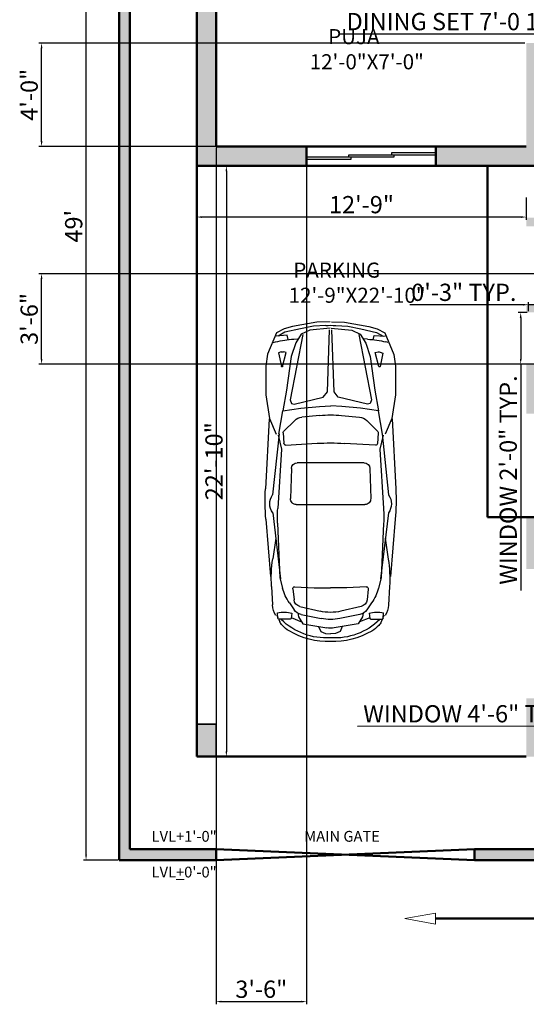
# Model space of a CAD drawing. Units: inches. Extents: x 1913 to 5309, y 1003 to 1733.
# Tile 13 of 23: x 3917 to 4152, y 1032 to 1489. Entities that reach past the tile are written whole.
import ezdxf

# ---------------------------------------------------------------- set-up
doc = ezdxf.new("R2010")
doc.units = ezdxf.units.IN
for name, color, linetype, lineweight in [('A-ANNO-DIMS', 2, 'Continuous', 18), ('A-ANNO-SYMB', 1, 'Continuous', 18), ('A-ANNO-TEXT', 7, 'Continuous', 18), ('A-AREA-IDEN', 3, 'Continuous', 18), ('A-COLS', 5, 'Continuous', 35), ('A-COLS-PATT', 5, 'Continuous', 13), ('A-EQPM', 8, 'Continuous', 18), ('A-FLOR-PATT', 252, 'Continuous', 13), ('A-GLAZ', 5, 'Continuous', 25), ('A-WALL', 7, 'Continuous', 50)]:
    doc.layers.add(name, color=color, linetype=linetype, lineweight=lineweight)
doc.layers.add('L9012X$0', color=2, linetype='Continuous')
doc.styles.get("Standard").update_dxf_attribs({"font": 'arial.ttf'})
doc.dimstyles.new('ISO-25', dxfattribs={"dimtxt": 8, "dimasz": 2.5, "dimexe": 1.25, "dimexo": 0.625, "dimtad": 1, "dimdec": 1, "dimlunit": 3, "dimtxsty": 'Standard', "dimcen": 2.5, "dimclrd": 256, "dimclrt": 1, "dimadec": 0, "dimazin": 0, "dimtfac": 1, "dimtdec": 1, "dimtmove": 0, "dimatfit": 3, "dimfxl": 1, "dimarcsym": 0})

# ---------------------------------------------------------------- blocks, each defined once
blk = doc.blocks.new('*D14')
at = {"layer": 'A-ANNO-DIMS', "color": 0, "lineweight": -2, "transparency": 16777216}
for p, q in [((3962.59, 1686.96), (3946.61, 1686.96)), ((3947.86, 1101.46), (3947.86, 1684.46)), ((3962.59, 1098.96), (3946.61, 1098.96))]:
    blk.add_line(p, q, dxfattribs=at)
at = {"layer": 'A-ANNO-DIMS', "color": 0, "transparency": 16777216}
for points in [[(3947.44, 1684.46), (3948.27, 1684.46), (3947.86, 1686.96)], [(3947.44, 1101.46), (3948.27, 1101.46), (3947.86, 1098.96)]]:
    blk.add_solid(points, dxfattribs=at)
at = {"layer": 'Defpoints', "color": 0, "transparency": 16777216}
for p in [(3947.86, 1686.96), (3963.21, 1686.96), (3963.21, 1098.96)]:
    blk.add_point(p, dxfattribs=at)
at = {"layer": 'A-ANNO-DIMS', "color": 0, "transparency": 16777216, "insert": (3943.15, 1392.96), "char_height": 8, "attachment_point": 5, "rotation": 90}
blk.add_mtext("49'", dxfattribs=at)
blk = doc.blocks.new('A1099DC')
at = {"color": 0, "linetype": 'ByBlock'}
for p, q in [((1279.298465, 804.448389), (2201.430588, 851.890505)), ((2602.736326, 846.078152), (3356.693814, 785.353187)), ((139.051458, 595.027331), (190.951238, 683.213377)), ((179.200345, 564.515703), (190.951238, 709.631982)), ((272.228253, 749.073842), (265.114727, 718.465169)), ((398.733388, 644.315148), (411.280494, 678.748261)), ((411.280494, 678.748261), (588.616917, 641.417897)), ((1482.852352, 674.283145), (1175.286956, 622.180789)), ((1475.52921, 670.226262), (2282.402739, 758.004075)), ((1494.603245, 682.841284), (1678.210958, 641.166865)), ((1678.210958, 641.166865), (2462.684993, 690.847736)), ((2519.280414, 756.817792), (3387.476361, 653.818028)), ((2656.476214, 692.831247), (3376.704709, 662.004075)), ((2851.341839, 715.213377), (3126.60716, 755.701993)), ((3376.704709, 662.004075), (3510.708679, 626.736433)), ((3488.458929, 772.663345), (3732.658862, 759.86454)), ((3909.27561, 688.812956), (3837.725727, 693.401722)), ((3867.794139, 700.329656), (3900.059395, 686.767505)), ((3921.162781, 527.618662), (3921.162781, 676.138994)), ((3925.383812, 676.122818), (3955.306409, 663.545364)), ((92.537504, 388.14361), (139.051458, 595.027331)), ((236.043912, 551.980927), (179.200345, 564.515703)), ((405.405047, 577.538958), (396.874865, 615.894428)), ((589.014326, 626.599587), (405.405047, 577.538958)), ((1300.814287, 466.658131), (1445.712032, 613.104998)), ((1465.665584, 620.56924), (1602.893878, 610.287296)), ((1626.354615, 583.507504), (1602.652901, 169.222264)), ((1933.148906, 509.557888), (2330.980062, 522.200075)), ((3704.596898, 536.993674), (3795.675135, 473.385795)), ((229.117398, 477.634662), (225.714299, 427.957563)), ((1860.238743, -448.635916), (1859.369151, 433.397797)), ((2409.60024, 445.938054), (2410.49349, -460.09121)), ((3493.960271, 465.734554), (3507.923021, 209.166865)), ((3522.252709, 492.345257), (3666.066199, 475.644444)), ((3753.293176, 397.789551), (3815.226005, 132.124765)), ((3839.396146, 426.841284), (3888.358202, 417.538958)), ((3841.786866, 503.451367), (3910.58243, 515.096797)), ((3888.358202, 417.538958), (3983.199613, 359.957848)), ((3901.001848, 514.780764), (3957.150905, 375.772812)), ((57.774444, 216.608726), (92.537504, 388.14361)), ((1235.045743, 136.116317), (1257.419842, 373.755108)), ((3857.610793, 379.525702), (3912.067615, 118.157673)), ((3983.199613, 359.957848), (4035.448301, 43.94997)), ((49.168662, 58.00681), (57.774444, 216.608726)), ((3507.923021, 209.166865), (3507.64153, -4.333678)), ((4019.086894, 150.376168), (4084.69605, 122.469191)), ((4084.69605, 122.469191), (4109.177079, 60.329656)), ((4109.177079, 60.329656), (4113.094043, -5.158716)), ((49.301278, -76.507426), (58.219773, -235.092064)), ((3508.347273, -221.154823), (3507.644805, -7.65525)), ((3858.370276, -390.823819), (3912.311631, -129.348921)), ((3983.920268, -371.008369), (4035.545755, -54.898082)), ((4084.948231, -133.320044), (4109.306686, -71.132359)), ((4109.306686, -71.132359), (4113.094514, -5.636391)), ((58.219773, -235.092064), (93.320996, -406.558069)), ((1235.330373, -152.586046), (1258.173002, -390.180259)), ((1627.520644, -599.204785), (1603.002095, -184.967086)), ((3494.890446, -477.749545), (3508.347273, -221.154823)), ((3754.088875, -409.293325), (3815.497749, -143.506937)), ((4019.394229, -161.356334), (4084.948231, -133.320044)), ((3889.19258, -428.776374), (3983.920268, -371.008369)), ((3902.027941, -525.993061), (3957.902795, -386.874665)), ((93.320996, -406.558069), (140.24279, -613.349673)), ((230.077082, -495.779641), (226.576036, -446.109349)), ((1301.750547, -482.997536), (1446.936772, -629.158411)), ((3523.2353, -504.304409), (3667.01558, -487.320059)), ((3705.667171, -548.593196), (3796.61981, -484.805853)), ((3840.248961, -438.175225), (3889.19258, -428.776374)), ((3842.790735, -514.780444), (3911.609128, -526.290202)), ((140.24279, -613.349673), (192.316354, -701.433212)), ((237.150178, -570.112104), (180.331436, -582.758939)), ((180.331436, -582.758939), (192.368445, -727.851766)), ((406.561378, -595.336142), (398.106841, -633.708356)), ((590.267037, -644.034637), (406.561378, -595.336142)), ((1484.19765, -690.263206), (1176.530118, -638.767405)), ((1466.905004, -636.583294), (1604.112757, -626.030785)), ((1934.168526, -524.650381), (2332.023837, -536.508105)), ((3378.022114, -674.249887), (3511.956283, -638.718087)), ((3922.214148, -538.79118), (3922.506998, -687.311224)), ((273.723073, -767.133288), (266.549207, -736.538701)), ((400.0214, -662.125356), (412.636377, -696.533662)), ((412.636377, -696.533662), (589.898847, -658.853701)), ((1476.866524, -686.22077), (2283.911563, -772.40743)), ((1495.965396, -698.798158), (1679.490579, -656.761786)), ((1679.490579, -656.761786), (2464.061049, -704.895745)), ((2520.786439, -770.754078), (3388.777604, -666.042617)), ((2657.855804, -706.497136), (3378.022114, -674.249887)), ((2852.765183, -728.494989), (3128.109803, -768.440762)), ((3489.994314, -784.688586), (3734.168535, -771.408296)), ((3910.644841, -700.0086), (3839.104145, -704.738438)), ((3869.186159, -711.60707), (3901.424611, -697.981326)), ((3926.727989, -687.286725), (3956.625729, -674.650294)), ((1280.900818, -820.829563), (2203.124693, -866.453338)), ((2604.418191, -859.849707), (3358.254477, -797.638217))]:
    blk.add_line(p, q, dxfattribs=at)
for points in [[(-0.000783, 0.794772), (5.385043, 172.701749), (63.649891, 493.818028), (92.537504, 603.957563), (144.437284, 705.166865), (428.417214, 824.236633), (585.095796, 846.190121), (961.406447, 846.190121), (1274.27399, 797.818028), (1482.852352, 709.631982)], [(83.345007, -3.206171), (111.32237, 268.957533), (164.563706, 379.583828), (279.999271, 453.709838), (456.549665, 511.628518), (901.254996, 574.918954), (1175.286956, 622.180789), (1137.52997, 385.548359), (1118.345181, 137.317882), (1109.829198, -8.358455)], [(168.178729, 359.003083), (1030.214866, 528.397865), (1077.798844, 510.531569), (1086.170082, 475.285426), (992.832238, 91.960378), (924.218938, 35.478085), (108.447994, 6.034416)], [(0.019119, -19.392451), (5.743899, -191.288474), (64.641806, -512.289243), (93.746535, -622.371603), (145.845778, -723.478374), (430.059935, -841.987962), (586.7815, -863.632471), (963.091723, -863.198028), (1275.863278, -814.209121), (1484.26735, -725.611974)], [(83.356858, -15.227176), (111.870816, -287.335185), (165.330179, -397.856284), (280.911681, -471.754535), (457.575935, -529.324983), (902.4055, -592.045995), (1176.530118, -638.767405), (1138.306616, -402.209884), (1118.632407, -154.017717), (1109.829198, -8.358455)], [(168.904615, -377.268451), (1031.273389, -545.270714), (1078.822046, -527.310627), (1087.123771, -492.048047), (993.030273, -108.907787), (924.305735, -52.560894), (108.478017, -24.418246)]]:
    blk.add_lwpolyline(points, dxfattribs=at)
for centre, radius, start, end in [((2358.037832, -2192.08357), 3048, 85.395244, 92.945173), ((2399.99649, 588.663508), 206.166238, 54.649181, 124.776949), ((1749.553982, 373.478072), 1524, 166.916578, 176.08111), ((2578.271641, -1134.295865), 1828.8, 87.549126, 93.623712), ((3392.740754, -1053.630025), 1828.8, 86.999806, 98.367602), ((3718.678317, 475.802507), 284.405862, 57.329946, 87.182375), ((4191.049821, 605.937201), 363.988953, 166.096081, 196.353514), ((3908.462781, 676.138994), 12.7, 0, 86.330429), ((3896.252417, 523.051998), 152.4, 46.38363, 67.20138), ((446.46332, 626.922805), 50.8, 159.97873, 192.538409), ((587.047263, 633.961317), 7.62, 284.960009, 78.112462), ((1463.767788, 595.240237), 25.4, 85.715073, 135.304647), ((1600.996082, 584.958293), 25.4, 356.725615, 85.715073), ((2333.400307, 446.03852), 76.2, 359.924458, 91.82012), ((3355.555414, 37.211519), 609.6, 55.070043, 75.255062), ((3908.462781, 527.618662), 12.7, 279.607718, 0), ((3320.85101, 50.338397), 847.430844, 356.245089, 44.519453), ((3700.933354, 318.064082), 435.542335, 30.457681, 46.38363), ((3204.184594, 25.950693), 1011.814461, 358.069446, 30.457681), ((1409.148822, 359.469565), 152.4, 135.304647, 174.62136), ((1935.569151, 433.396333), 76.2, 91.82012, 179.9989), ((3519.322741, 467.114813), 25.4, 83.37601, 183.115039), ((3654.346327, 374.722669), 101.6, 13.122645, 83.37601), ((3708.414764, 348.440256), 152.4, 11.769371, 55.070043), ((2752.335538, -6.739118), 1524, 174.62136, 185.491615), ((4645.676894, -4.872483), 3048, 176.725615, 183.38736), ((3221.54491, -6.276527), 609.6, 346.99033, 13.122645), ((1266.577845, -8.050136), 1219.2, 176.894161, 183.218814), ((3315.283499, -6.18411), 609.6, 348.343604, 11.769371), ((3734.73098, -5.770579), 304.8, 350.724636, 9.388339), ((3320.962449, -62.69553), 847.430844, 315.593523, 3.867886), ((3204.248172, -38.537915), 1011.814461, 329.655294, 2.043529), ((1750.305335, -388.625277), 1524, 184.031865, 193.196397), ((1409.873518, -375.595566), 152.4, 185.491615, 224.808328), ((1936.438592, -448.484202), 76.2, 180.114076, 268.292856), ((2334.293902, -460.341926), 76.2, 268.292856, 0.188517), ((3520.255588, -479.079792), 25.4, 176.997936, 276.736965), ((3655.096735, -386.42159), 101.6, 276.736965, 346.99033), ((3709.113243, -360.032616), 152.4, 305.042932, 348.343604), ((4192.255091, -616.577407), 363.988953, 163.759461, 194.016894), ((447.716945, -644.638934), 50.8, 167.574566, 200.134245), ((588.314493, -651.400231), 7.62, 282.000513, 75.152966), ((1464.957267, -611.258083), 25.4, 224.808328, 274.397903), ((1602.165021, -600.705574), 25.4, 274.397903, 3.38736), ((3355.640902, -49.500248), 609.6, 284.857913, 305.042932), ((3909.514173, -538.816222), 12.7, 0.112975, 80.505257), ((3897.294828, -534.273643), 152.4, 292.911596, 313.729345), ((3701.571953, -329.671253), 435.542335, 313.729345, 329.655294), ((2401.171182, -602.835323), 206.166238, 235.336026, 305.463794), ((2576.048678, 1120.472221), 1828.8, 266.489263, 272.563849), ((3390.675263, 1041.412497), 1828.8, 261.745373, 273.113169), ((3719.627907, -487.374382), 284.405862, 272.930601, 302.78303), ((3909.807023, -687.336265), 12.7, 273.782546, 0.112975), ((2353.729565, 2177.823616), 3048, 267.167802, 274.717731)]:
    blk.add_arc(centre, radius, start, end, dxfattribs=at)
blk = doc.blocks.new('VI')
at = {"layer": 'L9012X$0'}
blk.add_blockref('A1099DC', (0, 0), dxfattribs=at)
blk = doc.blocks.new('*D36')
at = {"layer": 'A-ANNO-DIMS', "color": 0, "lineweight": -2, "transparency": 16777216}
for p, q in [((3999.21, 1406.34), (3999.21, 1395.99)), ((4152.21, 1406.34), (4152.21, 1395.99)), ((4149.71, 1397.24), (4001.71, 1397.24))]:
    blk.add_line(p, q, dxfattribs=at)
at = {"layer": 'A-ANNO-DIMS', "color": 0, "transparency": 16777216}
for points in [[(4001.71, 1397.65), (4001.71, 1396.82), (3999.21, 1397.24)], [(4149.71, 1397.65), (4149.71, 1396.82), (4152.21, 1397.24)]]:
    blk.add_solid(points, dxfattribs=at)
at = {"layer": 'Defpoints', "color": 0, "transparency": 16777216}
for p in [(3999.21, 1406.96), (4152.21, 1406.96), (3999.21, 1397.24)]:
    blk.add_point(p, dxfattribs=at)
at = {"layer": 'A-ANNO-DIMS', "color": 0, "transparency": 16777216, "insert": (4075.71, 1401.95), "char_height": 8, "attachment_point": 5}
blk.add_mtext('12\'-9"', dxfattribs=at)
blk = doc.blocks.new('*D37')
at = {"layer": 'A-ANNO-DIMS', "color": 0, "lineweight": -2, "transparency": 16777216}
for p, q in [((4011.47, 1420.96), (4014.24, 1420.96)), ((4012.99, 1418.46), (4012.99, 1149.46)), ((4008.84, 1146.96), (4014.24, 1146.96))]:
    blk.add_line(p, q, dxfattribs=at)
at = {"layer": 'A-ANNO-DIMS', "color": 0, "transparency": 16777216}
for points in [[(4012.58, 1418.46), (4013.41, 1418.46), (4012.99, 1420.96)], [(4012.58, 1149.46), (4013.41, 1149.46), (4012.99, 1146.96)]]:
    blk.add_solid(points, dxfattribs=at)
at = {"layer": 'Defpoints', "color": 0, "transparency": 16777216}
for p in [(4010.85, 1420.96), (4008.21, 1146.96), (4012.99, 1146.96)]:
    blk.add_point(p, dxfattribs=at)
at = {"layer": 'A-ANNO-DIMS', "color": 0, "transparency": 16777216, "insert": (4008.28, 1283.96), "char_height": 8, "attachment_point": 5, "rotation": 90}
blk.add_mtext('22\'-10"', dxfattribs=at)
blk = doc.blocks.new('WIN-60')
for p, q in [((0, 60), (0, 39.5)), ((1, 60), (1, 19.5)), ((0, 39.5), (1, 39.5)), ((1, 40.5), (2, 40.5)), ((2, 40.5), (2, 0)), ((1, 19.5), (2, 19.5)), ((2, 20.5), (3, 20.5)), ((3, 20.5), (3, 0))]:
    blk.add_line(p, q)
blk = doc.blocks.new('*D57')
at = {"layer": 'A-ANNO-DIMS', "lineweight": -2, "transparency": 16777216}
for p, q in [((4178.83, 1161.04), (4073.85, 1160.96)), ((4230.33, 1161.08), (4181.33, 1161.05))]:
    blk.add_line(p, q, dxfattribs=at)
at = {"layer": 'A-ANNO-DIMS', "color": 0, "lineweight": -2, "transparency": 16777216}
for p, q in [((4178.84, 1153.57), (4178.83, 1162.29)), ((4232.84, 1153.61), (4232.83, 1162.33))]:
    blk.add_line(p, q, dxfattribs=at)
at = {"layer": 'A-ANNO-DIMS', "transparency": 16777216}
for points in [[(4181.33, 1161.46), (4181.33, 1160.63), (4178.83, 1161.04)], [(4230.33, 1161.5), (4230.33, 1160.67), (4232.83, 1161.08)]]:
    blk.add_solid(points, dxfattribs=at)
at = {"layer": 'Defpoints', "color": 0, "transparency": 16777216}
for p in [(4178.83, 1161.04), (4178.84, 1152.94), (4232.84, 1152.98)]:
    blk.add_point(p, dxfattribs=at)
at = {"layer": 'A-ANNO-DIMS', "color": 1, "transparency": 16777216, "insert": (4125.09, 1165.77), "char_height": 8, "attachment_point": 5, "rotation": 0.0441}
blk.add_mtext('WINDOW 4\'-6" TYP.', dxfattribs=at)
blk = doc.blocks.new('*D59')
at = {"layer": 'A-ANNO-DIMS', "color": 0, "lineweight": -2, "transparency": 16777216}
for p, q in [((4152.59, 1352.96), (4148.36, 1352.96)), ((4152.59, 1328.96), (4148.36, 1328.96))]:
    blk.add_line(p, q, dxfattribs=at)
at = {"layer": 'A-ANNO-DIMS', "lineweight": -2, "transparency": 16777216}
for p, q in [((4149.61, 1350.46), (4149.61, 1331.46)), ((4149.61, 1328.96), (4149.61, 1223.98))]:
    blk.add_line(p, q, dxfattribs=at)
at = {"layer": 'A-ANNO-DIMS', "transparency": 16777216}
for points in [[(4149.2, 1350.46), (4150.03, 1350.46), (4149.61, 1352.96)], [(4149.2, 1331.46), (4150.03, 1331.46), (4149.61, 1328.96)]]:
    blk.add_solid(points, dxfattribs=at)
at = {"layer": 'Defpoints', "color": 0, "transparency": 16777216}
for p in [(4153.21, 1352.96), (4149.61, 1328.96), (4153.21, 1328.96)]:
    blk.add_point(p, dxfattribs=at)
at = {"layer": 'A-ANNO-DIMS', "color": 1, "transparency": 16777216, "insert": (4144.85, 1275.22), "char_height": 8, "attachment_point": 5, "rotation": 90}
blk.add_mtext('WINDOW 2\'-0" TYP.', dxfattribs=at)
blk = doc.blocks.new('*D60')
at = {"layer": 'A-ANNO-DIMS', "lineweight": -2, "transparency": 16777216}
for p, q in [((4150.71, 1356.56), (4098.2, 1356.56)), ((4156.21, 1356.56), (4153.21, 1356.56)), ((4158.71, 1356.56), (4161.21, 1356.56))]:
    blk.add_line(p, q, dxfattribs=at)
at = {"layer": 'A-ANNO-DIMS', "color": 0, "lineweight": -2, "transparency": 16777216}
for p, q in [((4153.21, 1353.59), (4153.21, 1357.81)), ((4156.21, 1353.59), (4156.21, 1357.81))]:
    blk.add_line(p, q, dxfattribs=at)
at = {"layer": 'A-ANNO-DIMS', "transparency": 16777216}
for points in [[(4150.71, 1356.98), (4150.71, 1356.15), (4153.21, 1356.56)], [(4158.71, 1356.98), (4158.71, 1356.15), (4156.21, 1356.56)]]:
    blk.add_solid(points, dxfattribs=at)
at = {"layer": 'Defpoints', "color": 0, "transparency": 16777216}
for p in [(4153.21, 1356.56), (4153.21, 1352.96), (4156.21, 1352.96)]:
    blk.add_point(p, dxfattribs=at)
at = {"layer": 'A-ANNO-DIMS', "color": 1, "transparency": 16777216, "insert": (4123.21, 1361.28), "char_height": 8, "attachment_point": 5}
blk.add_mtext('0\'-3" TYP.', dxfattribs=at)
blk = doc.blocks.new('*D83')
at = {"layer": 'A-ANNO-DIMS', "lineweight": -2, "transparency": 16777216}
for p, q in [((4203.55, 1482.1), (4065.74, 1482.1)), ((4285.72, 1482.1), (4206.05, 1482.1))]:
    blk.add_line(p, q, dxfattribs=at)
at = {"layer": 'A-ANNO-DIMS', "color": 0, "lineweight": -2, "transparency": 16777216}
for p, q in [((4203.55, 1470.03), (4203.55, 1483.35)), ((4288.22, 1470.03), (4288.22, 1483.35))]:
    blk.add_line(p, q, dxfattribs=at)
at = {"layer": 'A-ANNO-DIMS', "transparency": 16777216}
for points in [[(4206.05, 1482.52), (4206.05, 1481.68), (4203.55, 1482.1)], [(4285.72, 1482.52), (4285.72, 1481.68), (4288.22, 1482.1)]]:
    blk.add_solid(points, dxfattribs=at)
at = {"layer": 'Defpoints', "color": 0, "transparency": 16777216}
for p in [(4203.55, 1482.1), (4203.55, 1469.4), (4288.22, 1469.4)]:
    blk.add_point(p, dxfattribs=at)
at = {"layer": 'A-ANNO-DIMS', "color": 1, "transparency": 16777216, "insert": (4133.4, 1486.86), "char_height": 8, "attachment_point": 5}
blk.add_mtext('DINING SET 7\'-0 1/2" TYP.', dxfattribs=at)
blk = doc.blocks.new('*D106')
at = {"layer": 'A-ANNO-DIMS', "color": 0, "lineweight": -2, "transparency": 16777216}
for p, q in [((4008.21, 1429.34), (4008.21, 1032.04)), ((4050.21, 1429.34), (4050.21, 1032.04))]:
    blk.add_line(p, q, dxfattribs=at)
at = {"layer": 'A-ANNO-DIMS', "lineweight": -2, "transparency": 16777216}
blk.add_line((4010.71, 1033.29), (4047.71, 1033.29), dxfattribs=at)
at = {"layer": 'A-ANNO-DIMS', "transparency": 16777216}
for points in [[(4010.71, 1033.7), (4010.71, 1032.87), (4008.21, 1033.29)], [(4047.71, 1033.7), (4047.71, 1032.87), (4050.21, 1033.29)]]:
    blk.add_solid(points, dxfattribs=at)
at = {"layer": 'Defpoints', "color": 0, "transparency": 16777216}
for p in [(4008.21, 1429.96), (4050.21, 1429.96), (4050.21, 1033.29)]:
    blk.add_point(p, dxfattribs=at)
at = {"layer": 'A-ANNO-DIMS', "color": 1, "transparency": 16777216, "insert": (4029.21, 1038), "char_height": 8, "attachment_point": 5}
blk.add_mtext('3\'-6"', dxfattribs=at)
blk = doc.blocks.new('*D109')
at = {"layer": 'A-ANNO-DIMS', "color": 0, "lineweight": -2, "transparency": 16777216}
for p, q in [((4151.59, 1477.96), (3925.96, 1477.96)), ((4151.59, 1429.96), (3925.96, 1429.96))]:
    blk.add_line(p, q, dxfattribs=at)
at = {"layer": 'A-ANNO-DIMS', "lineweight": -2, "transparency": 16777216}
blk.add_line((3927.21, 1432.46), (3927.21, 1475.46), dxfattribs=at)
at = {"layer": 'A-ANNO-DIMS', "transparency": 16777216}
for points in [[(3926.8, 1475.46), (3927.63, 1475.46), (3927.21, 1477.96)], [(3926.8, 1432.46), (3927.63, 1432.46), (3927.21, 1429.96)]]:
    blk.add_solid(points, dxfattribs=at)
at = {"layer": 'Defpoints', "color": 0, "transparency": 16777216}
for p in [(3927.21, 1477.96), (4152.21, 1477.96), (4152.21, 1429.96)]:
    blk.add_point(p, dxfattribs=at)
at = {"layer": 'A-ANNO-DIMS', "color": 1, "transparency": 16777216, "insert": (3922.5, 1453.96), "char_height": 8, "attachment_point": 5, "rotation": 90}
blk.add_mtext('4\'-0"', dxfattribs=at)
blk = doc.blocks.new('*D115')
at = {"layer": 'A-ANNO-DIMS', "color": 0, "lineweight": -2, "transparency": 16777216}
for p, q in [((4416.59, 1370.96), (3925.96, 1370.96)), ((4416.59, 1328.96), (3925.96, 1328.96))]:
    blk.add_line(p, q, dxfattribs=at)
at = {"layer": 'A-ANNO-DIMS', "lineweight": -2, "transparency": 16777216}
blk.add_line((3927.21, 1331.46), (3927.21, 1368.46), dxfattribs=at)
at = {"layer": 'A-ANNO-DIMS', "transparency": 16777216}
for points in [[(3926.8, 1368.46), (3927.63, 1368.46), (3927.21, 1370.96)], [(3926.8, 1331.46), (3927.63, 1331.46), (3927.21, 1328.96)]]:
    blk.add_solid(points, dxfattribs=at)
at = {"layer": 'Defpoints', "color": 0, "transparency": 16777216}
for p in [(3927.21, 1370.96), (4417.21, 1370.96), (4417.21, 1328.96)]:
    blk.add_point(p, dxfattribs=at)
at = {"layer": 'A-ANNO-DIMS', "color": 1, "transparency": 16777216, "insert": (3922.5, 1349.96), "char_height": 8, "attachment_point": 5, "rotation": 90}
blk.add_mtext('3\'-6"', dxfattribs=at)

msp = doc.modelspace()

# ---------------------------------------------------------------- hatches: boundary and pattern name
at = {"layer": 'A-COLS-PATT'}
h = msp.add_hatch(color=256, dxfattribs=at)
h.dxf.hatch_style = 1
h.paths.add_polyline_path([(3999.21, 1146.96), (4008.21, 1146.96), (4008.21, 1161.96), (3999.21, 1161.96)])
at = {"layer": 'A-FLOR-PATT'}
h = msp.add_hatch(color=256, dxfattribs=at)
h.dxf.hatch_style = 1
h.paths.add_polyline_path([(3968.21, 1681.96), (3999.21, 1681.96), (3999.21, 1686.96), (3963.21, 1686.96), (3963.21, 1098.96), (4008.21, 1098.96), (4008.21, 1103.96), (3968.21, 1103.96)])
h.paths.add_polyline_path([(4515.21, 1146.96), (4510.21, 1146.96), (4510.21, 1103.96), (4128.21, 1103.96), (4128.21, 1098.96), (4515.21, 1098.96)])
h = msp.add_hatch(color=256, dxfattribs=at)
h.dxf.hatch_style = 1
h.paths.add_polyline_path([(4179.21, 1155.93), (4164.35, 1155.93, -0.035946), (4163.9, 1155.96), (4161.21, 1155.96), (4161.21, 1173.96), (4152.21, 1173.96), (4152.21, 1146.96), (4179.21, 1146.96)])
h.paths.add_polyline_path([(4273.21, 1155.96), (4266.93, 1155.96), (4233.21, 1155.96), (4233.21, 1146.96), (4273.21, 1146.96)])
h.paths.add_polyline_path([(4285.21, 1328.96), (4152.21, 1328.96), (4152.21, 1305.96), (4161.21, 1305.96), (4161.21, 1323.96), (4285.21, 1323.96)])
h.paths.add_polyline_path([(4161.21, 1257.96), (4152.21, 1257.96), (4152.21, 1233.96), (4161.21, 1233.96), (4161.21, 1237.71)])
h.paths.add_polyline_path([(4515.21, 1405.96), (4503.21, 1405.96), (4503.21, 1400.96), (4506.21, 1400.96), (4506.21, 1328.96), (4452.21, 1328.96), (4452.21, 1323.96), (4506.21, 1323.96), (4506.21, 1179.96), (4455.21, 1179.96), (4455.21, 1170.96), (4515.21, 1170.96)])
h.paths.add_polyline_path([(4157.21, 1686.96), (3999.21, 1686.96), (3999.21, 1625.96), (4008.21, 1625.96), (4008.21, 1677.96), (4152.21, 1677.96), (4152.21, 1554.96), (4157.21, 1554.96), (4157.21, 1599.96), (4225.21, 1599.96), (4225.21, 1608.96), (4157.21, 1608.96)])
h.paths.add_polyline_path([(4008.21, 1513.96), (4157.21, 1513.96), (4157.21, 1518.96), (4008.21, 1518.96), (4008.21, 1571.96), (3999.21, 1571.96), (3999.21, 1420.96), (4050.21, 1420.96), (4050.21, 1429.96), (4008.21, 1429.96)])
h.paths.add_polyline_path([(4157.21, 1477.96), (4152.21, 1477.96), (4152.21, 1429.96), (4110.21, 1429.96), (4110.21, 1420.96), (4157.21, 1420.96)], flags=17)
h.paths.add_polyline_path([(4350.21, 1608.96), (4345.21, 1608.96), (4321.21, 1608.96), (4321.21, 1599.96), (4350.21, 1599.96)])
h.paths.add_polyline_path([(4515.21, 1686.96), (4345.21, 1686.96), (4345.21, 1644.96), (4350.21, 1644.96), (4350.21, 1677.96), (4506.21, 1677.96), (4506.21, 1557.96), (4423.21, 1557.96), (4423.21, 1552.96), (4506.21, 1552.96), (4506.21, 1492.96), (4428.21, 1492.96), (4428.21, 1522.96), (4423.21, 1522.96), (4423.21, 1492.96), (4345.21, 1492.96), (4345.21, 1487.96), (4474.21, 1487.96), (4474.21, 1464.96), (4479.21, 1464.96), (4479.21, 1487.96), (4515.21, 1487.96)])
h.paths.add_polyline_path([(4479.21, 1428.96), (4474.21, 1428.96), (4474.21, 1405.96), (4345.21, 1405.96), (4345.21, 1358.96), (4350.21, 1358.96), (4350.21, 1400.96), (4417.21, 1400.96), (4417.21, 1394.96), (4422.21, 1394.96), (4422.21, 1400.96), (4479.21, 1400.96)])
h.paths.add_polyline_path([(4350.21, 1323.96), (4422.21, 1323.96), (4422.21, 1370.96), (4417.21, 1370.96), (4417.21, 1328.96), (4345.21, 1328.96), (4345.21, 1158.97, -0.414214), (4342.21, 1155.96), (4327.21, 1155.96), (4327.21, 1146.96), (4350.21, 1146.96), (4350.21, 1170.96), (4401.21, 1170.96), (4401.21, 1179.96), (4350.21, 1179.96)])
h.paths.add_polyline_path([(4157.21, 1356.96), (4152.21, 1356.96), (4152.21, 1352.96), (4157.21, 1352.96)])
h.paths.add_polyline_path([(4157.21, 1396.96), (4152.21, 1396.96), (4152.21, 1392.96), (4157.21, 1392.96)])

# ---------------------------------------------------------------- linework, layer by layer
at = {"layer": 'A-ANNO-SYMB'}
msp.add_lwpolyline([(4095.87, 1071.84), (4110.03, 1074.39), (4110.03, 1069.29)], close=True, dxfattribs=at)
at = {"layer": 'A-COLS'}
msp.add_lwpolyline([(3999.21, 1146.96), (4008.21, 1146.96), (4008.21, 1161.96), (3999.21, 1161.96)], close=True, dxfattribs=at)
at = {"layer": 'A-WALL'}
for p, q in [((3963.21, 1098.96), (3963.21, 1686.96)), ((3999.21, 1686.96), (3999.21, 1420.96)), ((3968.21, 1103.96), (3968.21, 1681.96)), ((4008.21, 1513.96), (4008.21, 1429.96)), ((4008.21, 1429.96), (4152.21, 1429.96)), ((4050.21, 1420.96), (4050.21, 1429.96)), ((4110.21, 1420.96), (4110.21, 1429.96)), ((3999.21, 1420.96), (4157.21, 1420.96)), ((3999.21, 1420.96), (3999.21, 1146.96)), ((4134.21, 1420.96), (4134.21, 1257.96)), ((4134.21, 1257.96), (4161.21, 1257.96)), ((4152.21, 1146.96), (3999.21, 1146.96)), ((3968.21, 1103.96), (4008.21, 1103.96)), ((4008.21, 1103.96), (4008.21, 1098.96)), ((4008.21, 1103.96), (4128.21, 1098.96)), ((4008.21, 1098.96), (4128.21, 1103.96)), ((4128.21, 1103.96), (4128.21, 1098.96)), ((4128.21, 1103.96), (4510.21, 1103.96)), ((4008.21, 1098.96), (3963.21, 1098.96)), ((4515.21, 1098.96), (4128.21, 1098.96)), ((4110.03, 1071.84), (4209.85, 1071.84))]:
    msp.add_line(p, q, dxfattribs=at)

# ---------------------------------------------------------------- block references
at = {"layer": 'A-EQPM', "xscale": -0.0351896714874634, "yscale": 0.0351896714874634, "zscale": 0.0351896714874634, "rotation": 90}
msp.add_blockref('VI', (4061.12, 1348.67), dxfattribs=at)
at = {"layer": 'A-GLAZ', "rotation": 270.0000000000015}
msp.add_blockref('WIN-60', (4050.21, 1426.96), dxfattribs=at)

# ---------------------------------------------------------------- texts
at = {"layer": 'A-ANNO-TEXT', "char_height": 5, "attachment_point": 1}
for s, insert in [('{LVL+1\'-0"}', (3978.28, 1112.46)), ('{MAIN GATE}', (4049.16, 1112.46)), ('{LVL\\L+\\l0\'-0"}', (3978.28, 1095.88))]:
    msp.add_mtext_dynamic_manual_height_columns(s, width=86.9528, gutter_width=12.5, heights=[5.17], dxfattribs=dict(at, insert=insert))
at = {"layer": 'A-AREA-IDEN', "char_height": 7, "attachment_point": 1}
for s, insert in [('    PUJA\\P12\'-0"X7\'-0"', (4051.68, 1484.43)), (' PARKING\\P12\'-9"X22\'-10"', (4041.9, 1376.11))]:
    msp.add_mtext_dynamic_manual_height_columns(s, width=86.9528, gutter_width=12.5, heights=[0], dxfattribs=dict(at, insert=insert))

# ---------------------------------------------------------------- dimensions: what is measured, and where the dimension line sits
at = {"layer": 'A-ANNO-DIMS'}
for base, p1, p2, override, picture, middle in [((3947.86, 1686.96), (3963.21, 1098.96), (3963.21, 1686.96), {"dimclrd": 0, "dimclre": 0, "dimclrt": 0}, '*D14', (3943.15, 1392.96)), ((3927.21, 1477.96), (4152.21, 1429.96), (4152.21, 1477.96), {"dimdec": 1, "dimlfac": 1, "dimrnd": 0, "dimzin": 1, "dimdsep": 46, "dimlunit": 4, "dimfrac": 2}, '*D109', (3922.5, 1453.96)), ((4012.99, 1146.96), (4010.85, 1420.96), (4008.21, 1146.96), {"dimclrd": 0, "dimclre": 0, "dimclrt": 0}, '*D37', (4008.28, 1283.96)), ((3927.21, 1370.96), (4417.21, 1328.96), (4417.21, 1370.96), {"dimdec": 1, "dimlfac": 1, "dimrnd": 0, "dimzin": 1, "dimdsep": 46, "dimlunit": 4, "dimfrac": 2}, '*D115', (3922.5, 1349.96))]:
    dim = msp.add_linear_dim(base=base, p1=p1, p2=p2, angle=90, dimstyle='ISO-25', override=override, dxfattribs=at)
    dim.commit()
    dim.dimension.update_dxf_attribs({"geometry": picture, "text_midpoint": middle})
for base, p1, p2, angle, text, picture, middle in [((4203.55, 1482.1), (4288.22, 1469.4), (4203.55, 1469.4), 180, 'DINING SET <> TYP.', '*D83', (4133.4, 1486.86)), ((4153.21, 1356.56), (4156.21, 1352.96), (4153.21, 1352.96), 180, '<> TYP.', '*D60', (4123.21, 1361.28)), ((4149.61, 1328.96), (4153.21, 1352.96), (4153.21, 1328.96), 270, 'WINDOW <> TYP.', '*D59', (4144.85, 1275.22)), ((4178.83, 1161.04), (4232.84, 1152.98), (4178.84, 1152.94), 180.0441, 'WINDOW <> TYP.', '*D57', (4125.09, 1165.77))]:
    dim = msp.add_linear_dim(base=base, p1=p1, p2=p2, angle=angle, text=text, dimstyle='ISO-25', override={"dimdec": 1, "dimrnd": 0, "dimzin": 1, "dimlunit": 4, "dimfrac": 2}, dxfattribs=at)
    dim.commit()
    dim.dimension.update_dxf_attribs({"geometry": picture, "text_midpoint": middle})
for base, p1, p2, override, picture, middle in [((4050.21, 1033.29), (4008.21, 1429.96), (4050.21, 1429.96), {"dimdec": 1, "dimlfac": 1, "dimrnd": 0, "dimzin": 1, "dimdsep": 46, "dimlunit": 4, "dimfrac": 2}, '*D106', (4029.21, 1038)), ((3999.21, 1397.24), (4152.21, 1406.96), (3999.21, 1406.96), {"dimclrd": 0, "dimclre": 0, "dimclrt": 0}, '*D36', (4075.71, 1401.95))]:
    dim = msp.add_linear_dim(base=base, p1=p1, p2=p2, dimstyle='ISO-25', override=override, dxfattribs=at)
    dim.commit()
    dim.dimension.update_dxf_attribs({"geometry": picture, "text_midpoint": middle})

doc.saveas('drawing.dxf')
